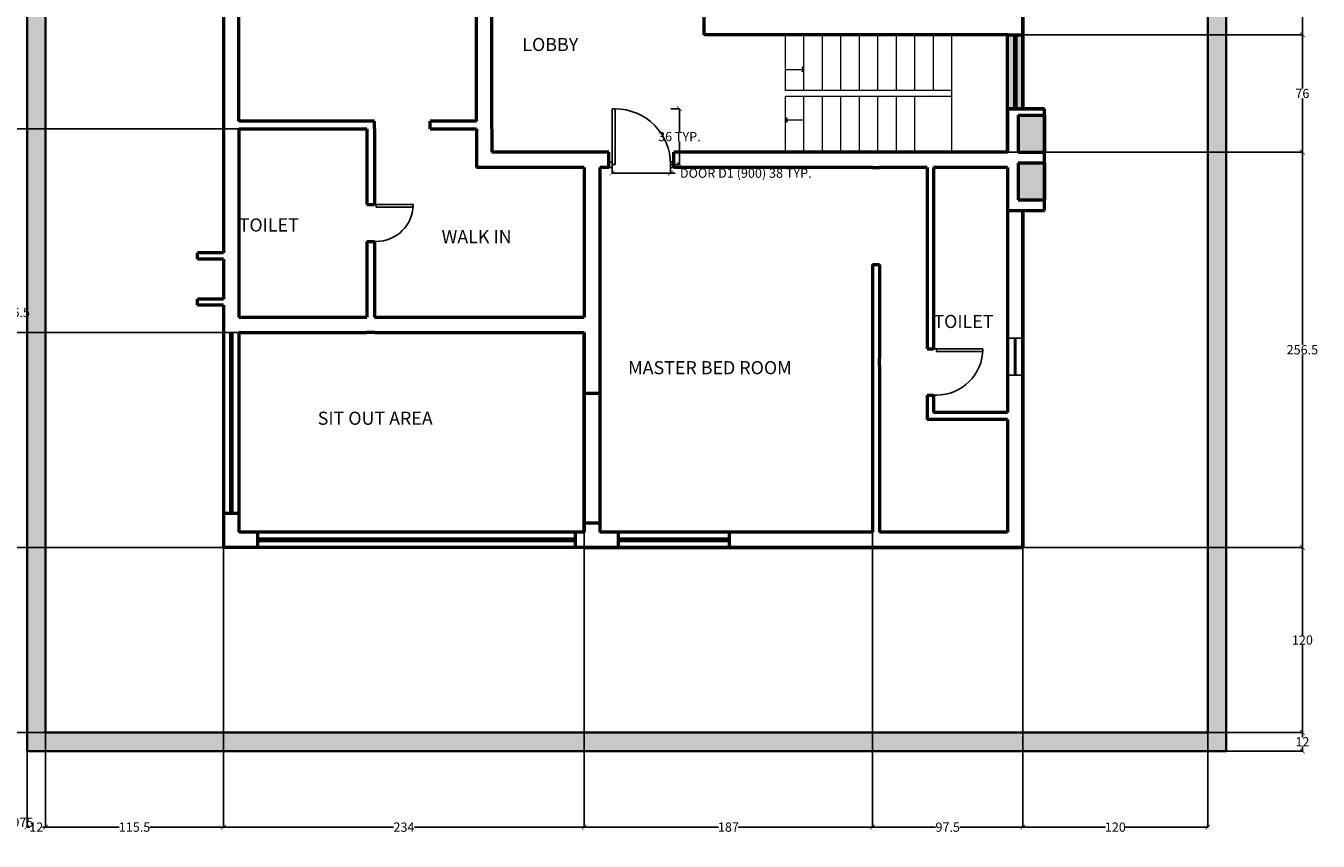
# Model space of a CAD drawing. Units: inches. Extents: x 925 to 2834, y 111 to 1355.
# Tile 24 of 25: x 1996 to 2834, y 170 to 699. Entities that reach past the tile are written whole.
import ezdxf

# ---------------------------------------------------------------- set-up
doc = ezdxf.new("R2010")
doc.units = ezdxf.units.IN
doc.header["$MEASUREMENT"] = 0
for name, color, linetype, lineweight in [('A-ANNO-DIMS', 2, 'Continuous', 18), ('A-ANNO-TTLB', 7, 'Continuous', 35), ('A-AREA-IDEN', 7, 'Continuous', 18), ('A-DOOR', 2, 'Continuous', 25), ('A-FLOR-PATT', 252, 'Continuous', 13), ('A-FLOR-STRS', 4, 'Continuous', 18), ('A-GLAZ', 3, 'Continuous', 25), ('A-WALL', 7, 'Continuous', 50), ('A-WALL-PATT', 8, 'Continuous', 13)]:
    doc.layers.add(name, color=color, linetype=linetype, lineweight=lineweight)
doc.styles.get("Standard").update_dxf_attribs({"font": 'arial.ttf'})
doc.dimstyles.get("Standard").update_dxf_attribs({"dimtxt": 6, "dimasz": 3, "dimexe": 0.18, "dimexo": 0.0625, "dimgap": 0.09, "dimtad": 0, "dimtih": 1, "dimtoh": 1, "dimdec": 1, "dimzin": 0, "dimdsep": 46, "dimlunit": 3, "dimtxsty": 'Standard', "dimblk": 'ARCHTICK', "dimcen": 0.09, "dimadec": 0, "dimazin": 0, "dimtfac": 1, "dimtdec": 1, "dimtofl": 0, "dimtmove": 0, "dimatfit": 3, "dimfxl": 1, "dimtolj": 1, "dimtzin": 0, "dimarcsym": 0})

# ---------------------------------------------------------------- blocks, each defined once
blk = doc.blocks.new('*U8')
for p, q in [((0, 0), (0, -6)), ((24, 0), (24, -6))]:
    blk.add_line(p, q)
blk.add_lwpolyline([(0, 0), (0, 24), (1.75, 24), (1.75, 0)], close=True)
blk.add_arc((0, 0), 24, 0, 90)
blk = doc.blocks.new('*U9')
for p, q in [((0, 0), (0, -6)), ((30, 0), (30, -6))]:
    blk.add_line(p, q)
blk.add_lwpolyline([(0, 0), (0, 30), (1.75, 30), (1.75, 0)], close=True)
blk.add_arc((0, 0), 30, 0, 90)
blk = doc.blocks.new('DOOR-900')
for p, q in [((0, 0), (0, 36)), ((0, 36), (2, 36)), ((2, 36), (2, 0)), ((2, 0), (0, 0))]:
    blk.add_line(p, q)
blk.add_arc((2, 0), 36, 0, 90)
blk = doc.blocks.new('_ArchTick')
at = {"color": 0, "linetype": 'ByBlock', "const_width": 0.15}
blk.add_lwpolyline([(-0.5, -0.5), (0.5, 0.5)], dxfattribs=at)
blk = doc.blocks.new('*D11')
at = {"layer": 'A-ANNO-DIMS', "color": 0, "lineweight": -2, "transparency": 16777216}
for p, q in [((2376.26, 609.33), (2376.26, 603.52)), ((2376.26, 603.7), (2414.26, 603.7)), ((2414.26, 609.33), (2414.26, 603.52)), ((2414.26, 603.7), (2417.26, 603.7))]:
    blk.add_line(p, q, dxfattribs=at)
at = {"layer": 'Defpoints', "color": 0, "transparency": 16777216}
for p in [(2376.26, 609.4), (2414.26, 609.4), (2414.26, 603.7)]:
    blk.add_point(p, dxfattribs=at)
at = {"layer": 'A-ANNO-DIMS', "color": 0, "lineweight": -2, "transparency": 16777216, "xscale": 3, "yscale": 3, "zscale": 3, "rotation": 180}
blk.add_blockref('_ArchTick', (2376.26, 603.7), dxfattribs=at)
at = {"layer": 'A-ANNO-DIMS', "color": 0, "lineweight": -2, "transparency": 16777216, "xscale": 3, "yscale": 3, "zscale": 3}
blk.add_blockref('_ArchTick', (2414.26, 603.7), dxfattribs=at)
at = {"layer": 'A-ANNO-DIMS', "color": 0, "transparency": 16777216, "insert": (2463.01, 603.7), "char_height": 6, "attachment_point": 5}
blk.add_mtext('\\A1;DOOR D1 (900) 38 TYP.', dxfattribs=at)
blk = doc.blocks.new('*D12')
at = {"layer": 'A-ANNO-DIMS', "color": 0, "lineweight": -2, "transparency": 16777216}
for p, q in [((2414.32, 645.4), (2420.14, 645.4)), ((2419.96, 645.4), (2419.96, 630.55)), ((2419.96, 609.4), (2419.96, 624.24)), ((2414.32, 609.4), (2420.14, 609.4))]:
    blk.add_line(p, q, dxfattribs=at)
at = {"layer": 'Defpoints', "color": 0, "transparency": 16777216}
for p in [(2414.26, 645.4), (2419.96, 645.4), (2414.26, 609.4)]:
    blk.add_point(p, dxfattribs=at)
at = {"layer": 'A-ANNO-DIMS', "color": 0, "lineweight": -2, "transparency": 16777216, "xscale": 3, "yscale": 3, "zscale": 3}
for p, rotation in [((2419.96, 645.4), 90), ((2419.96, 609.4), 270)]:
    blk.add_blockref('_ArchTick', p, dxfattribs=dict(at, rotation=rotation))
at = {"layer": 'A-ANNO-DIMS', "color": 0, "transparency": 16777216, "insert": (2419.96, 627.4), "char_height": 6, "attachment_point": 5}
blk.add_mtext('\\A1;36 TYP.', dxfattribs=at)
blk = doc.blocks.new('*D40')
at = {"layer": 'A-ANNO-DIMS', "color": 0, "lineweight": -2, "transparency": 16777216}
for p, q in [((1910.78, 193.09), (1988.62, 193.09)), ((1988.44, 193.09), (1988.44, 185.75)), ((1988.44, 172.11), (1988.44, 179.45)), ((1931.75, 172.11), (1988.62, 172.11))]:
    blk.add_line(p, q, dxfattribs=at)
at = {"layer": 'Defpoints', "color": 0, "transparency": 16777216}
for p in [(1910.71, 193.09), (1988.44, 193.09), (1931.69, 172.11)]:
    blk.add_point(p, dxfattribs=at)
at = {"layer": 'A-ANNO-DIMS', "color": 0, "lineweight": -2, "transparency": 16777216, "xscale": 3, "yscale": 3, "zscale": 3}
for p, rotation in [((1988.44, 193.09), 90), ((1988.44, 172.11), 270)]:
    blk.add_blockref('_ArchTick', p, dxfattribs=dict(at, rotation=rotation))
at = {"layer": 'A-ANNO-DIMS', "color": 0, "transparency": 16777216, "insert": (1988.44, 182.6), "char_height": 6, "attachment_point": 5}
blk.add_mtext('\\A1;20.975', dxfattribs=at)
blk = doc.blocks.new('*D44')
at = {"layer": 'A-ANNO-DIMS', "color": 0, "lineweight": -2, "transparency": 16777216}
for p, q in [((1708.78, 641.59), (1988.62, 641.59)), ((1988.44, 641.59), (1988.44, 516.49)), ((1988.44, 385.09), (1988.44, 510.19)), ((1718.78, 385.09), (1988.62, 385.09))]:
    blk.add_line(p, q, dxfattribs=at)
at = {"layer": 'Defpoints', "color": 0, "transparency": 16777216}
for p in [(1708.71, 641.59), (1988.44, 641.59), (1718.71, 385.09)]:
    blk.add_point(p, dxfattribs=at)
at = {"layer": 'A-ANNO-DIMS', "color": 0, "lineweight": -2, "transparency": 16777216, "xscale": 3, "yscale": 3, "zscale": 3}
for p, rotation in [((1988.44, 641.59), 90), ((1988.44, 385.09), 270)]:
    blk.add_blockref('_ArchTick', p, dxfattribs=dict(at, rotation=rotation))
at = {"layer": 'A-ANNO-DIMS', "color": 0, "transparency": 16777216, "insert": (1988.44, 513.34), "char_height": 6, "attachment_point": 5}
blk.add_mtext('\\A1;256.5', dxfattribs=at)
blk = doc.blocks.new('*D62')
at = {"layer": 'A-ANNO-DIMS', "color": 0, "lineweight": -2, "transparency": 16777216}
for p, q in [((2008.76, 240.83), (2008.76, 179.37)), ((1996.76, 228.83), (1996.76, 179.37)), ((1996.76, 179.55), (1998.68, 179.55)), ((2008.76, 179.55), (2006.83, 179.55))]:
    blk.add_line(p, q, dxfattribs=at)
at = {"layer": 'Defpoints', "color": 0, "transparency": 16777216}
for p in [(2008.76, 240.9), (1996.76, 228.9), (2008.76, 179.55)]:
    blk.add_point(p, dxfattribs=at)
at = {"layer": 'A-ANNO-DIMS', "color": 0, "lineweight": -2, "transparency": 16777216, "xscale": 3, "yscale": 3, "zscale": 3, "rotation": 180}
blk.add_blockref('_ArchTick', (1996.76, 179.55), dxfattribs=at)
at = {"layer": 'A-ANNO-DIMS', "color": 0, "lineweight": -2, "transparency": 16777216, "xscale": 3, "yscale": 3, "zscale": 3}
blk.add_blockref('_ArchTick', (2008.76, 179.55), dxfattribs=at)
at = {"layer": 'A-ANNO-DIMS', "color": 0, "transparency": 16777216, "insert": (2002.76, 179.55), "char_height": 6, "attachment_point": 5}
blk.add_mtext('\\A1;12', dxfattribs=at)
blk = doc.blocks.new('*D63')
at = {"layer": 'A-ANNO-DIMS', "color": 0, "lineweight": -2, "transparency": 16777216}
for p, q in [((2124.26, 360.83), (2124.26, 179.37)), ((2008.76, 240.83), (2008.76, 179.37)), ((2008.76, 179.55), (2056.55, 179.55)), ((2124.26, 179.55), (2076.46, 179.55))]:
    blk.add_line(p, q, dxfattribs=at)
at = {"layer": 'Defpoints', "color": 0, "transparency": 16777216}
for p in [(2124.26, 360.9), (2008.76, 240.9), (2124.26, 179.55)]:
    blk.add_point(p, dxfattribs=at)
at = {"layer": 'A-ANNO-DIMS', "color": 0, "lineweight": -2, "transparency": 16777216, "xscale": 3, "yscale": 3, "zscale": 3, "rotation": 180}
blk.add_blockref('_ArchTick', (2008.76, 179.55), dxfattribs=at)
at = {"layer": 'A-ANNO-DIMS', "color": 0, "lineweight": -2, "transparency": 16777216, "xscale": 3, "yscale": 3, "zscale": 3}
blk.add_blockref('_ArchTick', (2124.26, 179.55), dxfattribs=at)
at = {"layer": 'A-ANNO-DIMS', "color": 0, "transparency": 16777216, "insert": (2066.51, 179.55), "char_height": 6, "attachment_point": 5}
blk.add_mtext('\\A1;115.5', dxfattribs=at)
blk = doc.blocks.new('*D64')
at = {"layer": 'A-ANNO-DIMS', "color": 0, "lineweight": -2, "transparency": 16777216}
for p, q in [((2358.26, 370.83), (2358.26, 179.37)), ((2124.26, 360.83), (2124.26, 179.37)), ((2124.26, 179.55), (2234.5, 179.55)), ((2358.26, 179.55), (2248.02, 179.55))]:
    blk.add_line(p, q, dxfattribs=at)
at = {"layer": 'Defpoints', "color": 0, "transparency": 16777216}
for p in [(2358.26, 370.9), (2124.26, 360.9), (2358.26, 179.55)]:
    blk.add_point(p, dxfattribs=at)
at = {"layer": 'A-ANNO-DIMS', "color": 0, "lineweight": -2, "transparency": 16777216, "xscale": 3, "yscale": 3, "zscale": 3, "rotation": 180}
blk.add_blockref('_ArchTick', (2124.26, 179.55), dxfattribs=at)
at = {"layer": 'A-ANNO-DIMS', "color": 0, "lineweight": -2, "transparency": 16777216, "xscale": 3, "yscale": 3, "zscale": 3}
blk.add_blockref('_ArchTick', (2358.26, 179.55), dxfattribs=at)
at = {"layer": 'A-ANNO-DIMS', "color": 0, "transparency": 16777216, "insert": (2241.26, 179.55), "char_height": 6, "attachment_point": 5}
blk.add_mtext('\\A1;234', dxfattribs=at)
blk = doc.blocks.new('*D65')
at = {"layer": 'A-ANNO-DIMS', "color": 0, "lineweight": -2, "transparency": 16777216}
for p, q in [((2358.26, 370.83), (2358.26, 179.37)), ((2545.26, 370.83), (2545.26, 179.37)), ((2358.26, 179.55), (2445.32, 179.55)), ((2545.26, 179.55), (2458.19, 179.55))]:
    blk.add_line(p, q, dxfattribs=at)
at = {"layer": 'Defpoints', "color": 0, "transparency": 16777216}
for p in [(2358.26, 370.9), (2545.26, 370.9), (2545.26, 179.55)]:
    blk.add_point(p, dxfattribs=at)
at = {"layer": 'A-ANNO-DIMS', "color": 0, "lineweight": -2, "transparency": 16777216, "xscale": 3, "yscale": 3, "zscale": 3, "rotation": 180}
blk.add_blockref('_ArchTick', (2358.26, 179.55), dxfattribs=at)
at = {"layer": 'A-ANNO-DIMS', "color": 0, "lineweight": -2, "transparency": 16777216, "xscale": 3, "yscale": 3, "zscale": 3}
blk.add_blockref('_ArchTick', (2545.26, 179.55), dxfattribs=at)
at = {"layer": 'A-ANNO-DIMS', "color": 0, "transparency": 16777216, "insert": (2451.76, 179.55), "char_height": 6, "attachment_point": 5}
blk.add_mtext('\\A1;187', dxfattribs=at)
blk = doc.blocks.new('*D66')
at = {"layer": 'A-ANNO-DIMS', "color": 0, "lineweight": -2, "transparency": 16777216}
for p, q in [((2545.26, 370.83), (2545.26, 179.37)), ((2642.76, 360.83), (2642.76, 179.37)), ((2545.26, 179.55), (2586.1, 179.55)), ((2642.76, 179.55), (2601.91, 179.55))]:
    blk.add_line(p, q, dxfattribs=at)
at = {"layer": 'Defpoints', "color": 0, "transparency": 16777216}
for p in [(2545.26, 370.9), (2642.76, 360.9), (2642.76, 179.55)]:
    blk.add_point(p, dxfattribs=at)
at = {"layer": 'A-ANNO-DIMS', "color": 0, "lineweight": -2, "transparency": 16777216, "xscale": 3, "yscale": 3, "zscale": 3, "rotation": 180}
blk.add_blockref('_ArchTick', (2545.26, 179.55), dxfattribs=at)
at = {"layer": 'A-ANNO-DIMS', "color": 0, "lineweight": -2, "transparency": 16777216, "xscale": 3, "yscale": 3, "zscale": 3}
blk.add_blockref('_ArchTick', (2642.76, 179.55), dxfattribs=at)
at = {"layer": 'A-ANNO-DIMS', "color": 0, "transparency": 16777216, "insert": (2594.01, 179.55), "char_height": 6, "attachment_point": 5}
blk.add_mtext('\\A1;97.5', dxfattribs=at)
blk = doc.blocks.new('*D67')
at = {"layer": 'A-ANNO-DIMS', "color": 0, "lineweight": -2, "transparency": 16777216}
for p, q in [((2642.76, 360.83), (2642.76, 179.37)), ((2762.76, 240.83), (2762.76, 179.37)), ((2642.76, 179.55), (2696.33, 179.55)), ((2762.76, 179.55), (2709.18, 179.55))]:
    blk.add_line(p, q, dxfattribs=at)
at = {"layer": 'Defpoints', "color": 0, "transparency": 16777216}
for p in [(2642.76, 360.9), (2762.76, 240.9), (2762.76, 179.55)]:
    blk.add_point(p, dxfattribs=at)
at = {"layer": 'A-ANNO-DIMS', "color": 0, "lineweight": -2, "transparency": 16777216, "xscale": 3, "yscale": 3, "zscale": 3, "rotation": 180}
blk.add_blockref('_ArchTick', (2642.76, 179.55), dxfattribs=at)
at = {"layer": 'A-ANNO-DIMS', "color": 0, "lineweight": -2, "transparency": 16777216, "xscale": 3, "yscale": 3, "zscale": 3}
blk.add_blockref('_ArchTick', (2762.76, 179.55), dxfattribs=at)
at = {"layer": 'A-ANNO-DIMS', "color": 0, "transparency": 16777216, "insert": (2702.76, 179.55), "char_height": 6, "attachment_point": 5}
blk.add_mtext('\\A1;120', dxfattribs=at)
blk = doc.blocks.new('*D68')
at = {"layer": 'A-ANNO-DIMS', "color": 0, "lineweight": -2, "transparency": 16777216}
for p, q in [((2762.82, 240.9), (2824.29, 240.9)), ((2824.11, 240.9), (2824.11, 238)), ((2774.82, 228.9), (2824.29, 228.9)), ((2824.11, 228.9), (2824.11, 231.79))]:
    blk.add_line(p, q, dxfattribs=at)
at = {"layer": 'Defpoints', "color": 0, "transparency": 16777216}
for p in [(2762.76, 240.9), (2824.11, 240.9), (2774.76, 228.9)]:
    blk.add_point(p, dxfattribs=at)
at = {"layer": 'A-ANNO-DIMS', "color": 0, "lineweight": -2, "transparency": 16777216, "xscale": 3, "yscale": 3, "zscale": 3}
for p, rotation in [((2824.11, 240.9), 90), ((2824.11, 228.9), 270)]:
    blk.add_blockref('_ArchTick', p, dxfattribs=dict(at, rotation=rotation))
at = {"layer": 'A-ANNO-DIMS', "color": 0, "transparency": 16777216, "insert": (2824.11, 234.9), "char_height": 6, "attachment_point": 5}
blk.add_mtext('\\A1;12', dxfattribs=at)
blk = doc.blocks.new('*D69')
at = {"layer": 'A-ANNO-DIMS', "color": 0, "lineweight": -2, "transparency": 16777216}
for p, q in [((2642.82, 360.9), (2824.29, 360.9)), ((2824.11, 360.9), (2824.11, 304.05)), ((2824.11, 240.9), (2824.11, 297.74)), ((2762.82, 240.9), (2824.29, 240.9))]:
    blk.add_line(p, q, dxfattribs=at)
at = {"layer": 'Defpoints', "color": 0, "transparency": 16777216}
for p in [(2642.76, 360.9), (2824.11, 360.9), (2762.76, 240.9)]:
    blk.add_point(p, dxfattribs=at)
at = {"layer": 'A-ANNO-DIMS', "color": 0, "lineweight": -2, "transparency": 16777216, "xscale": 3, "yscale": 3, "zscale": 3}
for p, rotation in [((2824.11, 360.9), 90), ((2824.11, 240.9), 270)]:
    blk.add_blockref('_ArchTick', p, dxfattribs=dict(at, rotation=rotation))
at = {"layer": 'A-ANNO-DIMS', "color": 0, "transparency": 16777216, "insert": (2824.11, 300.9), "char_height": 6, "attachment_point": 5}
blk.add_mtext('\\A1;120', dxfattribs=at)
blk = doc.blocks.new('*D70')
at = {"layer": 'A-ANNO-DIMS', "color": 0, "lineweight": -2, "transparency": 16777216}
for p, q in [((2632.82, 617.4), (2824.29, 617.4)), ((2824.11, 617.4), (2824.11, 492.3)), ((2824.11, 360.9), (2824.11, 485.99)), ((2642.82, 360.9), (2824.29, 360.9))]:
    blk.add_line(p, q, dxfattribs=at)
at = {"layer": 'Defpoints', "color": 0, "transparency": 16777216}
for p in [(2632.76, 617.4), (2824.11, 617.4), (2642.76, 360.9)]:
    blk.add_point(p, dxfattribs=at)
at = {"layer": 'A-ANNO-DIMS', "color": 0, "lineweight": -2, "transparency": 16777216, "xscale": 3, "yscale": 3, "zscale": 3}
for p, rotation in [((2824.11, 617.4), 90), ((2824.11, 360.9), 270)]:
    blk.add_blockref('_ArchTick', p, dxfattribs=dict(at, rotation=rotation))
at = {"layer": 'A-ANNO-DIMS', "color": 0, "transparency": 16777216, "insert": (2824.11, 489.15), "char_height": 6, "attachment_point": 5}
blk.add_mtext('\\A1;256.5', dxfattribs=at)
blk = doc.blocks.new('*D71')
at = {"layer": 'A-ANNO-DIMS', "color": 0, "lineweight": -2, "transparency": 16777216}
for p, q in [((2632.82, 693.4), (2824.29, 693.4)), ((2824.11, 693.4), (2824.11, 658.55)), ((2824.11, 617.4), (2824.11, 652.24)), ((2632.82, 617.4), (2824.29, 617.4))]:
    blk.add_line(p, q, dxfattribs=at)
at = {"layer": 'Defpoints', "color": 0, "transparency": 16777216}
for p in [(2632.76, 693.4), (2824.11, 693.4), (2632.76, 617.4)]:
    blk.add_point(p, dxfattribs=at)
at = {"layer": 'A-ANNO-DIMS', "color": 0, "lineweight": -2, "transparency": 16777216, "xscale": 3, "yscale": 3, "zscale": 3}
for p, rotation in [((2824.11, 693.4), 90), ((2824.11, 617.4), 270)]:
    blk.add_blockref('_ArchTick', p, dxfattribs=dict(at, rotation=rotation))
at = {"layer": 'A-ANNO-DIMS', "color": 0, "transparency": 16777216, "insert": (2824.11, 655.4), "char_height": 6, "attachment_point": 5}
blk.add_mtext('\\A1;76', dxfattribs=at)
blk = doc.blocks.new('*D72')
at = {"layer": 'A-ANNO-DIMS', "color": 0, "lineweight": -2, "transparency": 16777216}
for p, q in [((2632.82, 953.4), (2824.29, 953.4)), ((2824.11, 953.4), (2824.11, 826.55)), ((2824.11, 693.4), (2824.11, 820.24)), ((2632.82, 693.4), (2824.29, 693.4))]:
    blk.add_line(p, q, dxfattribs=at)
at = {"layer": 'Defpoints', "color": 0, "transparency": 16777216}
for p in [(2632.76, 953.4), (2824.11, 953.4), (2632.76, 693.4)]:
    blk.add_point(p, dxfattribs=at)
at = {"layer": 'A-ANNO-DIMS', "color": 0, "lineweight": -2, "transparency": 16777216, "xscale": 3, "yscale": 3, "zscale": 3}
for p, rotation in [((2824.11, 953.4), 90), ((2824.11, 693.4), 270)]:
    blk.add_blockref('_ArchTick', p, dxfattribs=dict(at, rotation=rotation))
at = {"layer": 'A-ANNO-DIMS', "color": 0, "transparency": 16777216, "insert": (2824.11, 823.4), "char_height": 6, "attachment_point": 5}
blk.add_mtext('\\A1;260', dxfattribs=at)
blk = doc.blocks.new('*D75')
at = {"layer": 'A-ANNO-DIMS', "color": 0, "lineweight": -2, "transparency": 16777216}
for p, q in [((2124.2, 360.9), (1947.23, 360.9)), ((1947.41, 360.9), (1947.41, 304.05)), ((1947.41, 240.9), (1947.41, 297.74)), ((2008.7, 240.9), (1947.23, 240.9))]:
    blk.add_line(p, q, dxfattribs=at)
at = {"layer": 'Defpoints', "color": 0, "transparency": 16777216}
for p in [(1947.41, 360.9), (2124.26, 360.9), (2008.76, 240.9)]:
    blk.add_point(p, dxfattribs=at)
at = {"layer": 'A-ANNO-DIMS', "color": 0, "lineweight": -2, "transparency": 16777216, "xscale": 3, "yscale": 3, "zscale": 3}
for p, rotation in [((1947.41, 360.9), 90), ((1947.41, 240.9), 270)]:
    blk.add_blockref('_ArchTick', p, dxfattribs=dict(at, rotation=rotation))
at = {"layer": 'A-ANNO-DIMS', "color": 0, "transparency": 16777216, "insert": (1947.41, 300.9), "char_height": 6, "attachment_point": 5}
blk.add_mtext('\\A1;120', dxfattribs=at)
blk = doc.blocks.new('*D76')
at = {"layer": 'A-ANNO-DIMS', "color": 0, "lineweight": -2, "transparency": 16777216}
for p, q in [((2124.2, 500.4), (1947.23, 500.4)), ((1947.41, 500.4), (1947.41, 433.8)), ((1947.41, 360.9), (1947.41, 427.49)), ((2124.2, 360.9), (1947.23, 360.9))]:
    blk.add_line(p, q, dxfattribs=at)
at = {"layer": 'Defpoints', "color": 0, "transparency": 16777216}
for p in [(1947.41, 500.4), (2124.26, 500.4), (2124.26, 360.9)]:
    blk.add_point(p, dxfattribs=at)
at = {"layer": 'A-ANNO-DIMS', "color": 0, "lineweight": -2, "transparency": 16777216, "xscale": 3, "yscale": 3, "zscale": 3}
for p, rotation in [((1947.41, 500.4), 90), ((1947.41, 360.9), 270)]:
    blk.add_blockref('_ArchTick', p, dxfattribs=dict(at, rotation=rotation))
at = {"layer": 'A-ANNO-DIMS', "color": 0, "transparency": 16777216, "insert": (1947.41, 430.65), "char_height": 6, "attachment_point": 5}
blk.add_mtext('\\A1;139.5', dxfattribs=at)
blk = doc.blocks.new('*D77')
at = {"layer": 'A-ANNO-DIMS', "color": 0, "lineweight": -2, "transparency": 16777216}
for p, q in [((2134.2, 632.4), (1947.23, 632.4)), ((1947.41, 632.4), (1947.41, 569.55)), ((1947.41, 500.4), (1947.41, 563.24)), ((2124.2, 500.4), (1947.23, 500.4))]:
    blk.add_line(p, q, dxfattribs=at)
at = {"layer": 'Defpoints', "color": 0, "transparency": 16777216}
for p in [(1947.41, 632.4), (2134.26, 632.4), (2124.26, 500.4)]:
    blk.add_point(p, dxfattribs=at)
at = {"layer": 'A-ANNO-DIMS', "color": 0, "lineweight": -2, "transparency": 16777216, "xscale": 3, "yscale": 3, "zscale": 3}
for p, rotation in [((1947.41, 632.4), 90), ((1947.41, 500.4), 270)]:
    blk.add_blockref('_ArchTick', p, dxfattribs=dict(at, rotation=rotation))
at = {"layer": 'A-ANNO-DIMS', "color": 0, "transparency": 16777216, "insert": (1947.41, 566.4), "char_height": 6, "attachment_point": 5}
blk.add_mtext('\\A1;132', dxfattribs=at)
blk = doc.blocks.new('*D78')
at = {"layer": 'A-ANNO-DIMS', "color": 0, "lineweight": -2, "transparency": 16777216}
for p, q in [((2124.2, 808.4), (1947.23, 808.4)), ((1947.41, 808.4), (1947.41, 723.55)), ((1947.41, 632.4), (1947.41, 717.24)), ((2134.2, 632.4), (1947.23, 632.4))]:
    blk.add_line(p, q, dxfattribs=at)
at = {"layer": 'Defpoints', "color": 0, "transparency": 16777216}
for p in [(1947.41, 808.4), (2124.26, 808.4), (2134.26, 632.4)]:
    blk.add_point(p, dxfattribs=at)
at = {"layer": 'A-ANNO-DIMS', "color": 0, "lineweight": -2, "transparency": 16777216, "xscale": 3, "yscale": 3, "zscale": 3}
for p, rotation in [((1947.41, 808.4), 90), ((1947.41, 632.4), 270)]:
    blk.add_blockref('_ArchTick', p, dxfattribs=dict(at, rotation=rotation))
at = {"layer": 'A-ANNO-DIMS', "color": 0, "transparency": 16777216, "insert": (1947.41, 720.4), "char_height": 6, "attachment_point": 5}
blk.add_mtext('\\A1;176', dxfattribs=at)

msp = doc.modelspace()

# ---------------------------------------------------------------- hatches: boundary and pattern name
at = {"layer": 'A-FLOR-PATT'}
h = msp.add_hatch(color=256, dxfattribs=at)
h.dxf.hatch_style = 1
h.paths.add_polyline_path([(2774.758, 1189.3964), (1996.758, 1189.3964), (1996.758, 228.8964), (2774.758, 228.8964)])
h.paths.add_polyline_path([(2008.758, 1177.3964), (2762.758, 1177.3964), (2762.758, 240.8964), (2008.758, 240.8964)], flags=16)
h.paths.add_polyline_path([(2107.276, 551.9993), (2124.258, 551.9993), (2124.258, 703.3964), (2134.258, 703.3964), (2158.258, 703.3964), (2183.758, 703.3964), (2183.758, 751.3964), (2183.758, 775.3964), (2183.758, 823.3964), (2183.758, 969.395), (2183.758, 1041.395), (2183.758, 1047.3964), (2143.677, 1047.3964), (2143.677, 1057.3964), (2217.758, 1057.3964), (2265.758, 1057.3964), (2265.758, 1069.3964), (2271.758, 1069.3964), (2271.758, 1057.3964), (2295.758, 1057.3964), (2295.758, 1069.3964), (2301.758, 1069.3964), (2301.758, 1057.3964), (2592.758, 1057.3964), (2592.758, 1093.3964), (2599.758, 1093.3964), (2599.758, 1057.3964), (2635.758, 1057.3964), (2635.758, 1093.3964), (2642.758, 1093.3964), (2642.758, 1057.3964), (2642.758, 1025.9327), (2639.758, 1025.9327), (2639.758, 1001.9327), (2639.758, 977.9327), (2642.758, 977.9327), (2654.758, 977.9327), (2654.758, 973.9327), (2654.758, 965.9327), (2654.758, 961.9327), (2642.758, 961.9327), (2642.758, 869.3964), (2639.4187, 869.3964), (2639.4187, 867.3964), (2637.4187, 867.3964, 0.41421356), (2601.4187, 831.3964), (2637.4187, 831.3964), (2637.4187, 829.3964), (2639.4187, 829.3964), (2639.4187, 827.3964), (2642.758, 827.3964), (2642.758, 797.3943), (2658.5108, 797.3943), (2658.4187, 795.3964, -0.41421356), (2636.4868, 769.3964), (2636.4868, 767.3964), (2642.758, 767.3964), (2642.758, 693.3964), (2642.758, 645.3964), (2656.758, 645.3964), (2656.758, 641.3964), (2656.758, 617.3964), (2656.758, 610.3964), (2656.758, 586.3964), (2656.758, 579.3964), (2642.758, 579.3964), (2642.758, 360.8964), (2358.258, 360.8964), (2358.258, 408.8964), (2358.258, 506.3964), (2334.258, 506.3964), (2332.258, 506.3964), (2332.258, 508.3964, 0.41421356), (2296.258, 544.3964), (2296.258, 508.3964), (2294.258, 508.3964), (2294.258, 506.3964), (2292.258, 506.3964), (2206.258, 506.3964), (2134.258, 506.3964), (2124.258, 506.3964), (2124.258, 517.9993), (2107.276, 517.9993), (2107.276, 521.9993), (2124.258, 521.9993), (2124.258, 547.9993), (2107.276, 547.9993)], flags=0)
h.paths.add_polyline_path([(2134.258, 693.3964), (2134.258, 698.8964), (2158.258, 698.8964), (2158.258, 693.3964), (2368.258, 693.3964), (2368.258, 703.3964), (2193.758, 703.3964), (2188.258, 703.3964), (2188.258, 751.3964), (2193.758, 751.3964), (2193.758, 775.3964), (2188.258, 775.3964), (2188.258, 823.3964), (2193.758, 823.3964), (2193.758, 869.3964), (2193.758, 879.3964), (2193.758, 969.395), (2188.758, 969.395), (2188.758, 1005.395), (2189.758, 1005.395), (2189.758, 1041.395), (2193.758, 1041.395), (2193.758, 1047.3964), (2217.758, 1047.3964), (2217.758, 1052.8964), (2265.758, 1052.8964), (2265.758, 1051.8964), (2217.758, 1051.8964), (2217.758, 1047.3964), (2193.758, 1047.3964), (2193.758, 1041.395), (2190.758, 1041.395), (2190.758, 1005.395), (2189.758, 1005.395), (2189.758, 969.395), (2193.758, 969.395), (2193.758, 879.3964), (2193.758, 869.3964), (2193.758, 823.3964), (2189.258, 823.3964), (2189.258, 775.3964), (2193.758, 775.3964), (2193.758, 751.3964), (2189.258, 751.3964), (2189.258, 703.3964), (2193.758, 703.3964), (2368.258, 703.3964), (2368.258, 693.3964), (2158.258, 693.3964), (2158.258, 697.8964), (2134.258, 697.8964), (2134.258, 693.3964), (2134.258, 516.3964), (2134.258, 511.8964), (2206.258, 511.8964), (2206.258, 510.8964), (2134.258, 510.8964), (2134.258, 516.3964)], flags=0)
h.paths.add_polyline_path([(2374.258, 610.7178), (2376.258, 610.7178), (2376.258, 645.3964), (2378.258, 645.3964, -0.40021217), (2414.2165, 611.1251), (2416.258, 611.1251), (2416.258, 617.3964), (2488.758, 617.3964), (2488.758, 653.3964), (2596.758, 653.3964), (2596.758, 657.3964), (2488.758, 657.3964), (2488.758, 693.3964), (2435.758, 693.3964), (2435.758, 723.8964), (2435.758, 747.8964), (2435.758, 775.3964), (2435.758, 833.3964), (2435.9366, 833.3964), (2435.9366, 835.3964), (2439.6653, 835.3964, 0.41421356), (2461.5973, 855.3964), (2437.5973, 855.3964), (2435.9366, 855.3964), (2435.9366, 857.3964), (2435.758, 857.3964), (2435.758, 869.3964), (2375.758, 869.3964), (2375.758, 879.3964), (2516.758, 879.3964), (2516.758, 914.3964), (2516.758, 916.3964), (2520.4868, 916.3964, 0.41421356), (2542.4187, 942.3964), (2518.4187, 942.3964), (2516.758, 942.3964), (2516.758, 944.3964), (2520.0795, 944.3964), (2526.758, 944.3964), (2632.758, 944.3964), (2632.758, 879.3964), (2526.758, 879.3964), (2526.758, 914.3964), (2516.758, 914.3964), (2516.758, 879.3964), (2375.758, 879.3964), (2375.758, 869.3964), (2435.758, 869.3964), (2435.758, 857.3964), (2442.758, 857.3964), (2442.758, 869.3964), (2516.758, 869.3964), (2516.758, 775.3964), (2442.758, 775.3964), (2442.758, 833.3964), (2435.758, 833.3964), (2435.758, 775.3964), (2435.758, 747.8964), (2445.758, 747.8964), (2445.758, 768.3964), (2516.758, 768.3964), (2516.758, 703.3964), (2445.758, 703.3964), (2445.758, 723.8964), (2435.758, 723.8964), (2435.758, 693.3964), (2632.758, 693.3964), (2638.258, 693.3964), (2638.258, 645.3964), (2632.758, 645.3964), (2632.758, 617.3964), (2416.258, 617.3964), (2416.258, 607.3964), (2545.258, 607.3964), (2545.258, 418.8964), (2549.758, 418.8964), (2549.758, 478.8964), (2549.758, 483.3964), (2549.758, 607.3964), (2632.758, 607.3964), (2632.758, 483.3964), (2579.758, 483.3964), (2579.758, 478.8964), (2632.758, 478.8964), (2632.758, 370.8964), (2549.758, 370.8964), (2549.758, 394.8964), (2545.258, 394.8964), (2545.258, 370.8964), (2406.258, 370.8964), (2406.258, 364.8964), (2362.258, 364.8964), (2362.258, 367.6686), (2362.258, 408.8964), (2368.258, 408.8964), (2368.258, 607.3964), (2374.258, 607.3964)], flags=0)
h.paths.add_polyline_path([(2368.258, 408.8964), (2368.258, 370.8964), (2406.258, 370.8964), (2406.258, 366.8964), (2364.258, 366.8964), (2364.258, 367.6686), (2364.258, 408.8964)], flags=0)
h.paths.add_polyline_path([(2229.758, 869.3964), (2229.758, 879.3964), (2301.758, 879.3964), (2301.758, 869.3964)], flags=0)
h.paths.add_polyline_path([(2488.758, 638.1212), (2489.8812, 639.6555), (2489.5021, 638.621), (2490.027, 638.1212), (2489.5021, 637.6214), (2489.8812, 636.5869)], flags=0)
h.paths.add_polyline_path([(2499.4891, 671.007), (2500.014, 671.5068), (2499.6349, 672.5413), (2500.758, 671.007), (2499.6349, 669.4727), (2500.014, 670.5072)], flags=0)
h.paths.add_polyline_path([(2632.758, 797.3964), (2636.0795, 797.3964), (2636.0795, 795.3964), (2634.4187, 795.3964), (2632.758, 795.3964)], flags=0)
at = {"layer": 'A-WALL-PATT', "transparency": 33554605}
h = msp.add_hatch(color=256, dxfattribs=at)
h.dxf.hatch_style = 1
h.paths.add_polyline_path([(2656.758, 610.3964), (2639.758, 610.3964), (2639.758, 586.3964), (2656.758, 586.3964)])
h.paths.add_polyline_path([(2656.758, 641.3964), (2639.758, 641.3964), (2639.758, 617.3964), (2656.758, 617.3964)])
h.paths.add_polyline_path([(2654.758, 973.9327), (2642.758, 973.9327), (2642.758, 965.9327), (2654.758, 965.9327)])
at = {"layer": 'A-WALL-PATT'}
h = msp.add_hatch(color=256, dxfattribs=at)
h.dxf.hatch_style = 1
h.set_gradient(color1=(255, 255, 255), tint=1)
h.paths.add_polyline_path([(2642.758, 645.3964), (2642.758, 693.3964), (2638.258, 693.3964), (2638.258, 645.3964)])
h.paths.add_polyline_path([(2637.258, 645.3964), (2637.258, 693.3964), (2632.758, 693.3964), (2632.758, 645.3964)])
h = msp.add_hatch(color=256, dxfattribs=at)
h.dxf.hatch_style = 1
h.set_gradient(color1=(99, 100, 102), color2=(99, 100, 102), tint=1)
h.paths.add_polyline_path([(2638.258, 645.3964), (2638.258, 693.3964), (2637.258, 693.3964), (2637.258, 645.3964)])

# ---------------------------------------------------------------- linework, layer by layer
at = {"layer": 'A-ANNO-TTLB'}
for p, q in [((1996.758, 1189.3964), (1996.758, 228.8964)), ((2774.758, 228.8964), (2774.758, 1189.3964)), ((2008.758, 1177.3964), (2008.758, 240.8964)), ((2762.758, 1177.3964), (2762.758, 240.8964)), ((2762.758, 240.8964), (2762.758, 1177.3964)), ((2762.758, 240.8964), (2762.758, 1057.3964)), ((2008.758, 506.3964), (2008.758, 240.8964)), ((2762.758, 240.8964), (2008.758, 240.8964)), ((2008.758, 240.8964), (2384.258, 240.8964)), ((2008.758, 240.8964), (2762.758, 240.8964)), ((2358.258, 240.8964), (2762.758, 240.8964)), ((1996.758, 228.8964), (2774.758, 228.8964))]:
    msp.add_line(p, q, dxfattribs=at)
at = {"layer": 'A-DOOR'}
for points in [[(2374.258, 610.7178), (2376.258, 610.7178), (2376.258, 607.3964), (2374.258, 607.3964)], [(2414.258, 611.1251), (2416.258, 611.1251), (2416.258, 607.3964), (2414.258, 607.3964)]]:
    msp.add_lwpolyline(points, close=True, dxfattribs=at)
at = {"layer": 'A-FLOR-STRS'}
for p, q in [((2488.758, 657.3964), (2488.758, 693.3964)), ((2500.758, 657.3964), (2500.758, 693.3964)), ((2512.758, 657.3964), (2512.758, 693.3964)), ((2524.758, 657.3964), (2524.758, 693.3964)), ((2536.758, 657.3964), (2536.758, 693.3964)), ((2548.758, 657.3964), (2548.758, 693.3964)), ((2560.758, 657.3964), (2560.758, 693.3964)), ((2572.758, 657.3964), (2572.758, 693.3964)), ((2584.758, 657.3964), (2584.758, 693.3964)), ((2596.758, 617.3964), (2596.758, 693.3964)), ((2488.758, 671.007), (2499.4891, 671.007)), ((2500.014, 671.5068), (2499.4891, 671.007)), ((2500.014, 670.5072), (2499.4891, 671.007)), ((2500.758, 671.007), (2499.6349, 672.5413)), ((2499.6349, 672.5413), (2500.014, 671.5068)), ((2500.758, 671.007), (2499.6349, 669.4727)), ((2499.6349, 669.4727), (2500.014, 670.5072)), ((2596.758, 657.3964), (2488.758, 657.3964)), ((2596.758, 653.3964), (2488.758, 653.3964)), ((2488.758, 617.3964), (2488.758, 653.3964)), ((2500.758, 617.3964), (2500.758, 653.3964)), ((2512.758, 617.3964), (2512.758, 653.3964)), ((2524.758, 617.3964), (2524.758, 653.3964)), ((2536.758, 617.3964), (2536.758, 653.3964)), ((2548.758, 617.3964), (2548.758, 653.3964)), ((2560.758, 617.3964), (2560.758, 653.3964)), ((2572.758, 617.3964), (2572.758, 653.3964)), ((2488.758, 638.1212), (2489.8812, 639.6555)), ((2488.758, 638.1212), (2489.8812, 636.5869)), ((2489.8812, 639.6555), (2489.5021, 638.621)), ((2489.5021, 638.621), (2490.027, 638.1212)), ((2489.5021, 637.6214), (2490.027, 638.1212)), ((2489.8812, 636.5869), (2489.5021, 637.6214)), ((2500.758, 638.1212), (2490.027, 638.1212))]:
    msp.add_line(p, q, dxfattribs=at)
at = {"layer": 'A-GLAZ'}
for p, q in [((2128.258, 500.3423), (2128.258, 382.8964)), ((2129.258, 500.3423), (2129.258, 382.8964)), ((2130.258, 500.3423), (2130.258, 382.8964)), ((2637.258, 496.576), (2637.258, 472.576)), ((2637.758, 496.576), (2637.758, 472.576)), ((2638.258, 496.576), (2638.258, 472.576)), ((2146.258, 366.8964), (2352.258, 366.8964)), ((2146.258, 365.8964), (2352.258, 365.8964)), ((2146.258, 364.8964), (2352.258, 364.8964)), ((2380.258, 366.8964), (2452.258, 366.8964)), ((2380.258, 365.8964), (2452.258, 365.8964)), ((2380.258, 364.8964), (2452.258, 364.8964))]:
    msp.add_line(p, q, dxfattribs=at)
for points in [[(2134.258, 500.3423), (2134.258, 382.8964), (2124.258, 382.8964), (2124.258, 500.3423)], [(2642.758, 496.576), (2642.758, 472.576), (2632.758, 472.576), (2632.758, 496.576)], [(2146.258, 370.8964), (2352.258, 370.8964), (2352.258, 360.8964), (2146.258, 360.8964)], [(2380.258, 370.8964), (2452.258, 370.8964), (2452.258, 360.8964), (2380.258, 360.8964)]]:
    msp.add_lwpolyline(points, close=True, dxfattribs=at)
at = {"layer": 'A-WALL'}
for p, q in [((2642.758, 645.3964), (2642.758, 961.9327)), ((2124.258, 808.3964), (2124.258, 551.9993)), ((2134.258, 637.3964), (2134.258, 798.3964)), ((2288.258, 637.3964), (2288.258, 798.3964)), ((2298.258, 632.3964), (2298.258, 798.3964)), ((2642.758, 767.3964), (2642.758, 693.3964)), ((2435.758, 723.8964), (2435.758, 693.3964)), ((2642.758, 703.3964), (2642.758, 693.3964)), ((2632.758, 693.3964), (2435.758, 693.3964)), ((2632.758, 693.3964), (2642.758, 693.3964)), ((2632.758, 617.3964), (2632.758, 693.3964)), ((2637.258, 693.3964), (2637.258, 645.3964)), ((2638.258, 693.3964), (2638.258, 645.3964)), ((2222.258, 637.3964), (2134.258, 637.3964)), ((2222.258, 632.3964), (2222.258, 637.3964)), ((2288.258, 637.3964), (2258.258, 637.3964)), ((2258.258, 632.3964), (2258.258, 637.3964)), ((2632.758, 645.3964), (2632.758, 617.3964)), ((2632.758, 645.3964), (2642.758, 645.3964)), ((2632.758, 645.3964), (2656.758, 645.3964)), ((2639.758, 641.3964), (2639.758, 617.3964)), ((2639.758, 641.3964), (2656.758, 641.3964)), ((2656.758, 645.3964), (2642.758, 645.3964)), ((2656.758, 641.3964), (2656.758, 645.3964)), ((2656.758, 579.3964), (2656.758, 645.3964)), ((2656.758, 641.3964), (2656.758, 617.3964)), ((2134.258, 632.3964), (2217.258, 632.3964)), ((2134.258, 632.3964), (2134.258, 516.3964)), ((2217.258, 632.3964), (2217.258, 583.3964)), ((2222.258, 632.3964), (2222.258, 583.3964)), ((2258.258, 632.3964), (2288.258, 632.3964)), ((2288.258, 632.3964), (2288.258, 607.3964)), ((2298.258, 632.3964), (2298.258, 617.3964)), ((2358.258, 617.3964), (2298.258, 617.3964)), ((2374.258, 617.3964), (2358.258, 617.3964)), ((2374.258, 607.3964), (2374.258, 617.3964)), ((2632.758, 617.3964), (2416.258, 617.3964)), ((2416.258, 607.3964), (2416.258, 617.3964)), ((2639.758, 617.3964), (2656.758, 617.3964)), ((2656.758, 610.3964), (2656.758, 617.3964)), ((2358.258, 607.3964), (2288.258, 607.3964)), ((2358.258, 607.3964), (2358.258, 510.3964)), ((2374.258, 607.3964), (2368.258, 607.3964)), ((2368.258, 607.3964), (2368.258, 370.8964)), ((2545.258, 607.3964), (2416.258, 607.3964)), ((2545.258, 607.3964), (2549.758, 607.3964)), ((2580.758, 607.3964), (2549.758, 607.3964)), ((2580.758, 607.3964), (2580.758, 489.6926)), ((2632.758, 607.3964), (2584.758, 607.3964)), ((2584.758, 607.3964), (2584.758, 489.6926)), ((2632.758, 607.3964), (2632.758, 483.3964)), ((2639.758, 610.3964), (2639.758, 586.3964)), ((2639.758, 610.3964), (2656.758, 610.3964)), ((2656.758, 610.3964), (2656.758, 586.3964)), ((2217.258, 583.3964), (2222.258, 583.3964)), ((2632.758, 579.3964), (2632.758, 448.3964)), ((2632.758, 579.3964), (2656.758, 579.3964)), ((2639.758, 586.3964), (2656.758, 586.3964)), ((2642.758, 579.3964), (2642.758, 360.8964)), ((2642.758, 360.8964), (2642.758, 579.3964)), ((2642.758, 579.3964), (2656.758, 579.3964)), ((2656.758, 579.3964), (2656.758, 586.3964)), ((2217.258, 559.3964), (2222.258, 559.3964)), ((2217.258, 559.3964), (2217.258, 510.3964)), ((2222.258, 559.3964), (2222.258, 516.3964)), ((2124.258, 551.9993), (2107.276, 551.9993)), ((2107.276, 547.9993), (2107.276, 551.9993)), ((2124.258, 547.9993), (2107.276, 547.9993)), ((2124.258, 547.9993), (2124.258, 521.9993)), ((2545.258, 544.3964), (2545.258, 370.8964)), ((2545.258, 544.3964), (2549.758, 544.3964)), ((2549.758, 544.3964), (2549.758, 483.3964)), ((2124.258, 521.9993), (2107.276, 521.9993)), ((2107.276, 517.9993), (2107.276, 521.9993)), ((2124.258, 517.9993), (2107.276, 517.9993)), ((2124.258, 517.9993), (2124.258, 510.3151)), ((2134.258, 516.3964), (2134.258, 510.3964)), ((2222.258, 516.3964), (2222.258, 510.3964)), ((2124.258, 510.3151), (2124.258, 500.3964)), ((2134.258, 510.3964), (2217.258, 510.3964)), ((2222.258, 510.3964), (2358.258, 510.3964)), ((2124.258, 500.3964), (2124.258, 360.8964)), ((2134.258, 500.3964), (2217.258, 500.3964)), ((2134.258, 500.3964), (2134.258, 370.8964)), ((2222.258, 500.3964), (2217.258, 500.3964)), ((2222.258, 500.3964), (2358.258, 500.3964)), ((2358.258, 500.3964), (2358.258, 370.8964)), ((2358.258, 370.8964), (2358.258, 500.3964)), ((2580.758, 489.6926), (2584.758, 489.6926)), ((2549.758, 478.8964), (2549.758, 483.3964)), ((2549.758, 478.8964), (2549.758, 370.8964)), ((2358.258, 460.8964), (2368.258, 460.8964)), ((2580.758, 459.6926), (2584.758, 459.6926)), ((2580.758, 459.6926), (2580.758, 443.8964)), ((2584.758, 459.6926), (2584.758, 448.3964)), ((2632.758, 448.3964), (2584.758, 448.3964)), ((2632.758, 443.8964), (2580.758, 443.8964)), ((2632.758, 443.8964), (2632.758, 370.8964)), ((2545.258, 394.8964), (2545.258, 370.8964)), ((2549.758, 394.8964), (2549.758, 370.8964)), ((2134.258, 382.8964), (2124.258, 382.8964)), ((2358.258, 370.8964), (2134.258, 370.8964)), ((2146.258, 370.8964), (2146.258, 360.8964)), ((2352.258, 370.8964), (2352.258, 360.8964)), ((2358.258, 376.8964), (2368.258, 376.8964)), ((2545.258, 370.8964), (2368.258, 370.8964)), ((2380.258, 370.8964), (2380.258, 360.8964)), ((2452.258, 370.8964), (2452.258, 360.8964)), ((2632.758, 370.8964), (2549.758, 370.8964)), ((2358.258, 360.8964), (2124.258, 360.8964)), ((2642.758, 360.8964), (2358.258, 360.8964)), ((2384.258, 360.8964), (2358.258, 360.8964)), ((2358.258, 360.8964), (2638.0452, 360.8964)), ((2638.0452, 360.8964), (2642.758, 360.8964))]:
    msp.add_line(p, q, dxfattribs=at)
msp.add_lwpolyline([(2642.758, 693.3964), (2642.758, 645.3964), (2632.758, 645.3964), (2632.758, 693.3964)], close=True, dxfattribs=at)

# ---------------------------------------------------------------- block references
at = {"layer": 'A-DOOR'}
msp.add_blockref('DOOR-900', (2376.2583, 609.3968), dxfattribs=at)
at = {"layer": 'A-DOOR', "rotation": 270}
for name, p in [('*U8', (2223.258, 583.3964)), ('*U9', (2586.758, 489.6926))]:
    msp.add_blockref(name, p, dxfattribs=at)

# ---------------------------------------------------------------- texts
at = {"layer": 'A-AREA-IDEN'}
for s, height, p in [('LOBBY', 8.49473, (2318.08, 682.8977)), ('TOILET', 8.49473, (2134.094, 565.8381)), ('WALK IN', 8.49473, (2265.7255, 558.2665)), ('TOILET', 8.49473, (2584.758, 503.2566)), ('MASTER BED ROOM', 8.494735, (2386.7437, 473.2934)), ('SIT OUT AREA', 8.494735, (2185.3493, 440.4902))]:
    msp.add_text(s, height=height, dxfattribs=at).set_placement(p)

# ---------------------------------------------------------------- dimensions: what is measured, and where the dimension line sits
at = {"layer": 'A-ANNO-DIMS'}
for base, p1, p2, override, picture, middle in [((2824.108, 953.3964), (2632.758, 693.3964), (2632.758, 953.3964), {"dimdec": 0, "dimlfac": 1, "dimrnd": 0, "dimzin": 0, "dimdsep": 46, "dimlunit": 2}, '*D72', (2824.108, 823.3964)), ((1947.408, 808.3964), (2134.258, 632.3964), (2124.258, 808.3964), {"dimdec": 0, "dimlfac": 1, "dimrnd": 0, "dimzin": 0, "dimdsep": 46, "dimlunit": 2}, '*D78', (1947.408, 720.3964)), ((2824.108, 693.3964), (2632.758, 617.3964), (2632.758, 693.3964), {"dimdec": 0, "dimlfac": 1, "dimrnd": 0, "dimzin": 0, "dimdsep": 46, "dimlunit": 2}, '*D71', (2824.108, 655.3964)), ((1988.438, 641.5886), (1718.7128, 385.0886), (1708.7128, 641.5886), {"dimdec": 1, "dimlfac": 1, "dimrnd": 0, "dimzin": 0, "dimdsep": 46, "dimlunit": 2}, '*D44', (1988.438, 513.3386)), ((1947.408, 632.3964), (2124.258, 500.3964), (2134.258, 632.3964), {"dimdec": 0, "dimlfac": 1, "dimrnd": 0, "dimzin": 0, "dimdsep": 46, "dimlunit": 2}, '*D77', (1947.408, 566.3964)), ((2824.108, 617.3964), (2642.758, 360.8964), (2632.758, 617.3964), {"dimdec": 1, "dimlfac": 1, "dimrnd": 0, "dimzin": 0, "dimdsep": 46, "dimlunit": 2}, '*D70', (2824.108, 489.1464)), ((1947.408, 500.3964), (2124.258, 360.8964), (2124.258, 500.3964), {"dimdec": 1, "dimlfac": 1, "dimrnd": 0, "dimzin": 0, "dimdsep": 46, "dimlunit": 2}, '*D76', (1947.408, 430.6464)), ((1947.408, 360.8964), (2008.758, 240.8964), (2124.258, 360.8964), {"dimdec": 0, "dimlfac": 1, "dimrnd": 0, "dimzin": 0, "dimdsep": 46, "dimlunit": 2}, '*D75', (1947.408, 300.8964)), ((2824.108, 360.8964), (2762.758, 240.8964), (2642.758, 360.8964), {"dimdec": 0, "dimlfac": 1, "dimrnd": 0, "dimzin": 0, "dimdsep": 46, "dimlunit": 2}, '*D69', (2824.108, 300.8964)), ((2824.108, 240.8964), (2774.758, 228.8964), (2762.758, 240.8964), {"dimdec": 0, "dimlfac": 1, "dimrnd": 0, "dimzin": 0, "dimdsep": 46, "dimlunit": 2}, '*D68', (2824.108, 234.8964)), ((1988.438, 193.0886), (1931.688, 172.1134), (1910.7128, 193.0886), {"dimdec": 3, "dimlfac": 1, "dimrnd": 0, "dimzin": 0, "dimdsep": 46, "dimlunit": 2}, '*D40', (1988.438, 182.601))]:
    dim = msp.add_linear_dim(base=base, p1=p1, p2=p2, angle=90, dimstyle='Standard', override=override, dxfattribs=at)
    dim.commit()
    dim.dimension.update_dxf_attribs({"geometry": picture, "text_midpoint": middle})
dim = msp.add_linear_dim(base=(2419.958, 645.3964), p1=(2414.258, 609.3964), p2=(2414.258, 645.3964), angle=90, text='<> TYP.', dimstyle='Standard', override={"dimdec": 0, "dimrnd": 0, "dimzin": 0, "dimlunit": 2}, dxfattribs=at)
dim.commit()
dim.dimension.update_dxf_attribs({"geometry": '*D12', "text_midpoint": (2419.958, 627.3964)})
dim = msp.add_linear_dim(base=(2414.258, 603.6964), p1=(2376.258, 609.3964), p2=(2414.258, 609.3964), text='DOOR D1 (900) <> TYP.', dimstyle='Standard', override={"dimdec": 0, "dimrnd": 0, "dimzin": 0, "dimlunit": 2}, dxfattribs=at)
dim.commit()
dim.dimension.update_dxf_attribs({"geometry": '*D11', "text_midpoint": (2463.009, 603.6964)})
for base, p1, p2, override, picture, middle in [((2358.258, 179.5464), (2124.258, 360.8964), (2358.258, 370.8964), {"dimdec": 0, "dimlfac": 1, "dimrnd": 0, "dimzin": 0, "dimdsep": 46, "dimlunit": 2}, '*D64', (2241.258, 179.5464)), ((2545.258, 179.5464), (2358.258, 370.8964), (2545.258, 370.8964), {"dimdec": 0, "dimlfac": 1, "dimrnd": 0, "dimzin": 0, "dimdsep": 46, "dimlunit": 2}, '*D65', (2451.758, 179.5464)), ((2642.758, 179.5464), (2545.258, 370.8964), (2642.758, 360.8964), {"dimdec": 1, "dimlfac": 1, "dimrnd": 0, "dimzin": 0, "dimdsep": 46, "dimlunit": 2}, '*D66', (2594.008, 179.5464)), ((2124.258, 179.5464), (2008.758, 240.8964), (2124.258, 360.8964), {"dimdec": 1, "dimlfac": 1, "dimrnd": 0, "dimzin": 0, "dimdsep": 46, "dimlunit": 2}, '*D63', (2066.508, 179.5464)), ((2762.758, 179.5464), (2642.758, 360.8964), (2762.758, 240.8964), {"dimdec": 0, "dimlfac": 1, "dimrnd": 0, "dimzin": 0, "dimdsep": 46, "dimlunit": 2}, '*D67', (2702.758, 179.5464)), ((2008.758, 179.5464), (1996.758, 228.8964), (2008.758, 240.8964), {"dimdec": 0, "dimlfac": 1, "dimrnd": 0, "dimzin": 0, "dimdsep": 46, "dimlunit": 2}, '*D62', (2002.758, 179.5464))]:
    dim = msp.add_linear_dim(base=base, p1=p1, p2=p2, dimstyle='Standard', override=override, dxfattribs=at)
    dim.commit()
    dim.dimension.update_dxf_attribs({"geometry": picture, "text_midpoint": middle})

doc.saveas('drawing.dxf')
